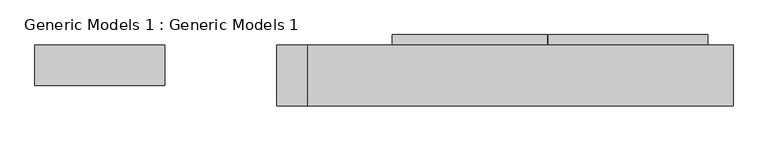
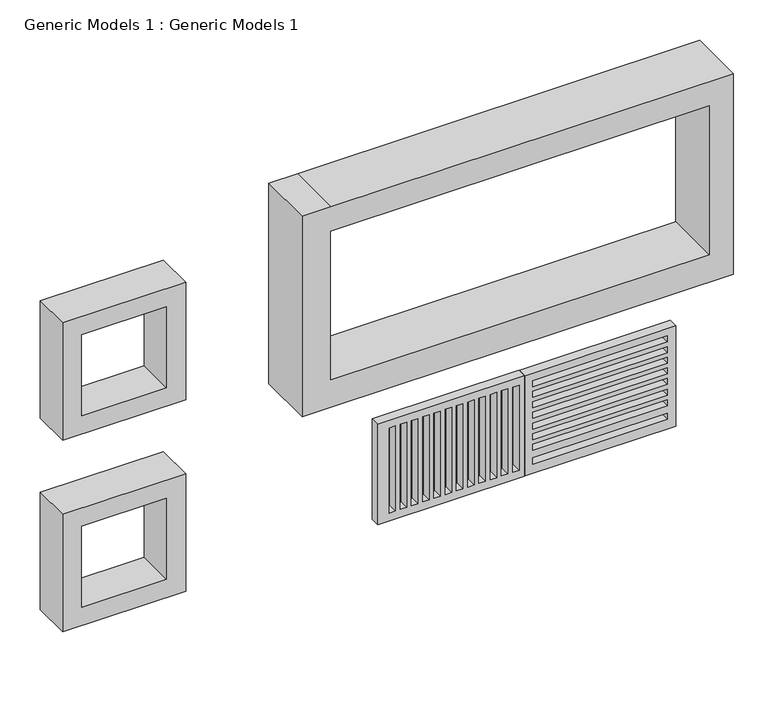
"""IFC4 building model written with IfcOpenShell, lengths in millimetres: proxy geometry, Generic Models 1 : Generic Models 1."""

from ifc_helpers import new_model, si_unit, frame, origin, place, context, project, spatial, polyline, outline, extrude, source, transform, mapped, element, save


def generic_models_1_generic_models_1_e6b78f1d(model_context):
    return source(origin(), model_context, "Body", "SweptSolid", [
        extrude(outline(polyline([(82.3687651, 4516.4585096), (1760.22, 4516.4585096), (1760.22, 2136.8093783), (82.3687651, 2136.8093783), (82.3687651, 4516.4585096)]), holes=[polyline([(1535.9752881, 2253.5343465), (1637.5752881, 2253.5343465), (1637.5752881, 4387.1343465), (1535.9752881, 4387.1343465), (1535.9752881, 2253.5343465)]), polyline([(1358.1752881, 2253.5343465), (1459.7752881, 2253.5343465), (1459.7752881, 4387.1343465), (1358.1752881, 4387.1343465), (1358.1752881, 2253.5343465)]), polyline([(1180.3752881, 2253.5343465), (1281.9752881, 2253.5343465), (1281.9752881, 4387.1343465), (1180.3752881, 4387.1343465), (1180.3752881, 2253.5343465)]), polyline([(1002.5752881, 2253.5343465), (1104.1752881, 2253.5343465), (1104.1752881, 4387.1343465), (1002.5752881, 4387.1343465), (1002.5752881, 2253.5343465)]), polyline([(824.7752881, 2253.5343465), (926.3752881, 2253.5343465), (926.3752881, 4387.1343465), (824.7752881, 4387.1343465), (824.7752881, 2253.5343465)]), polyline([(646.9752881, 2253.5343465), (748.5752881, 2253.5343465), (748.5752881, 4387.1343465), (646.9752881, 4387.1343465), (646.9752881, 2253.5343465)]), polyline([(469.1752881, 2253.5343465), (570.7752881, 2253.5343465), (570.7752881, 4387.1343465), (469.1752881, 4387.1343465), (469.1752881, 2253.5343465)]), polyline([(240.5752881, 2253.5343465), (342.1752881, 2253.5343465), (342.1752881, 4387.1343465), (240.5752881, 4387.1343465), (240.5752881, 2253.5343465)])]), frame((0.0, -9654.1523906, 0.0), z_axis=(0.0, 1.0, 0.0), x_axis=(0.0, 0.0, 1.0)), (0.0, 0.0, 1.0), 152.4),
        extrude(outline(polyline([(1760.22, -195.2414904), (82.3687651, -195.2414904), (82.3687651, 2119.6486563), (1760.22, 2119.6486563), (1760.22, -195.2414904)]), holes=[polyline([(215.1752881, -18.7817081), (1637.5752881, -18.7817081), (1637.5752881, 82.8182919), (215.1752881, 82.8182919), (215.1752881, -18.7817081)]), polyline([(215.1752881, 159.0182919), (1637.5752881, 159.0182919), (1637.5752881, 260.6182919), (215.1752881, 260.6182919), (215.1752881, 159.0182919)]), polyline([(215.1752881, 336.8182919), (1637.5752881, 336.8182919), (1637.5752881, 438.4182919), (215.1752881, 438.4182919), (215.1752881, 336.8182919)]), polyline([(215.1752881, 514.6182919), (1637.5752881, 514.6182919), (1637.5752881, 616.2182919), (215.1752881, 616.2182919), (215.1752881, 514.6182919)]), polyline([(215.1752881, 692.4182919), (1637.5752881, 692.4182919), (1637.5752881, 794.0182919), (215.1752881, 794.0182919), (215.1752881, 692.4182919)]), polyline([(215.1752881, 870.2182919), (1637.5752881, 870.2182919), (1637.5752881, 971.8182919), (215.1752881, 971.8182919), (215.1752881, 870.2182919)]), polyline([(215.1752881, 1048.0182919), (1637.5752881, 1048.0182919), (1637.5752881, 1149.6182919), (215.1752881, 1149.6182919), (215.1752881, 1048.0182919)]), polyline([(215.1752881, 1225.8182919), (1637.5752881, 1225.8182919), (1637.5752881, 1327.4182919), (215.1752881, 1327.4182919), (215.1752881, 1225.8182919)]), polyline([(215.1752881, 1403.6182919), (1637.5752881, 1403.6182919), (1637.5752881, 1505.2182919), (215.1752881, 1505.2182919), (215.1752881, 1403.6182919)]), polyline([(215.1752881, 1581.4182919), (1637.5752881, 1581.4182919), (1637.5752881, 1683.0182919), (215.1752881, 1683.0182919), (215.1752881, 1581.4182919)]), polyline([(215.1752881, 1759.2182919), (1637.5752881, 1759.2182919), (1637.5752881, 1860.8182919), (215.1752881, 1860.8182919), (215.1752881, 1759.2182919)]), polyline([(215.1752881, 1937.0182919), (1637.5752881, 1937.0182919), (1637.5752881, 2038.6182919), (215.1752881, 2038.6182919), (215.1752881, 1937.0182919)])]), frame((0.0, -9654.1523906, 0.0), z_axis=(0.0, 1.0, 0.0), x_axis=(0.0, 0.0, 1.0)), (0.0, 0.0, 1.0), 152.4),
        extrude(outline(polyline([(5695.95, -3590.1102404), (5695.95, -5533.2102404), (3730.6676291, -5533.2102404), (3730.6676291, -3590.1102404), (5695.95, -3590.1102404)]), holes=[polyline([(5391.15, -3894.9102404), (4035.4676291, -3894.9102404), (4035.4676291, -5228.4102404), (5391.15, -5228.4102404), (5391.15, -3894.9102404)])]), frame((0.0, -10263.7523906, 0.0), z_axis=(0.0, 1.0, 0.0), x_axis=(0.0, 0.0, 1.0)), (0.0, 0.0, 1.0), 609.6),
        extrude(outline(polyline([(2495.55, -3590.1102404), (2495.55, -5533.2102404), (530.2676291, -5533.2102404), (530.2676291, -3590.1102404), (2495.55, -3590.1102404)]), holes=[polyline([(2190.75, -3894.9102404), (835.0676291, -3894.9102404), (835.0676291, -5228.4102404), (2190.75, -5228.4102404), (2190.75, -3894.9102404)])]), frame((0.0, -10263.7523906, 0.0), z_axis=(0.0, 1.0, 0.0), x_axis=(0.0, 0.0, 1.0)), (0.0, 0.0, 1.0), 609.6),
        extrude(outline(polyline([(6400.8, -1465.2414904), (6400.8, -1922.4414904), (3048.0, -1922.4414904), (3048.0, -1465.2414904), (3048.0, 4897.4585096), (3505.2, 4897.4585096), (6400.8, 4897.4585096), (6400.8, -1465.2414904)]), holes=[polyline([(3505.2, -1465.2414904), (5994.4, -1465.2414904), (5994.4, 4516.4585096), (3505.2, 4516.4585096), (3505.2, -1465.2414904)])]), frame((0.0, -10568.5523906, 0.0), z_axis=(0.0, 1.0, 0.0), x_axis=(0.0, 0.0, 1.0)), (0.0, 0.0, 1.0), 914.4),
    ])


if __name__ == "__main__":
    model = new_model("IFC4")
    model_context = context("Model", 3, world=origin())
    ifc_project = project(units=[si_unit("LENGTHUNIT", "METRE", prefix="MILLI")], contexts=[model_context])
    site = spatial("IfcSite", under=ifc_project)
    building = spatial("IfcBuilding", under=site)
    placement = place(None, origin())
    generic_models_1_generic_models_1_shape = generic_models_1_generic_models_1_e6b78f1d(model_context)
    element("IfcBuildingElementProxy", 1, Name="Generic Models 1 : Generic Models 1", ObjectType="Generic Models 1 : Generic Models 1", at=placement, inside=building, context=model_context, shape_type="MappedRepresentation", body=[
        mapped(generic_models_1_generic_models_1_shape, transform((0.0, 0.0, 0.0), x_axis=(1.0, 0.0, 0.0), y_axis=(0.0, 1.0, 0.0), z_axis=(0.0, 0.0, 1.0))),
    ])
    save(model, "model.ifc")

# Revit data of these elements
# Element 1 (IfcBuildingElementProxy, "Generic Models 1 : Generic Models 1")
#   Materials on its faces: "Wood Planks", "wood 1"
# Materials
#   "Wood Planks": class "Wood", colour RGB 193 160 115, transparency 0, Description = "Physical material.", Cost = 0
#   "wood 1": class "Generic", colour RGB 51 32 15, transparency 0, Cost = 0
